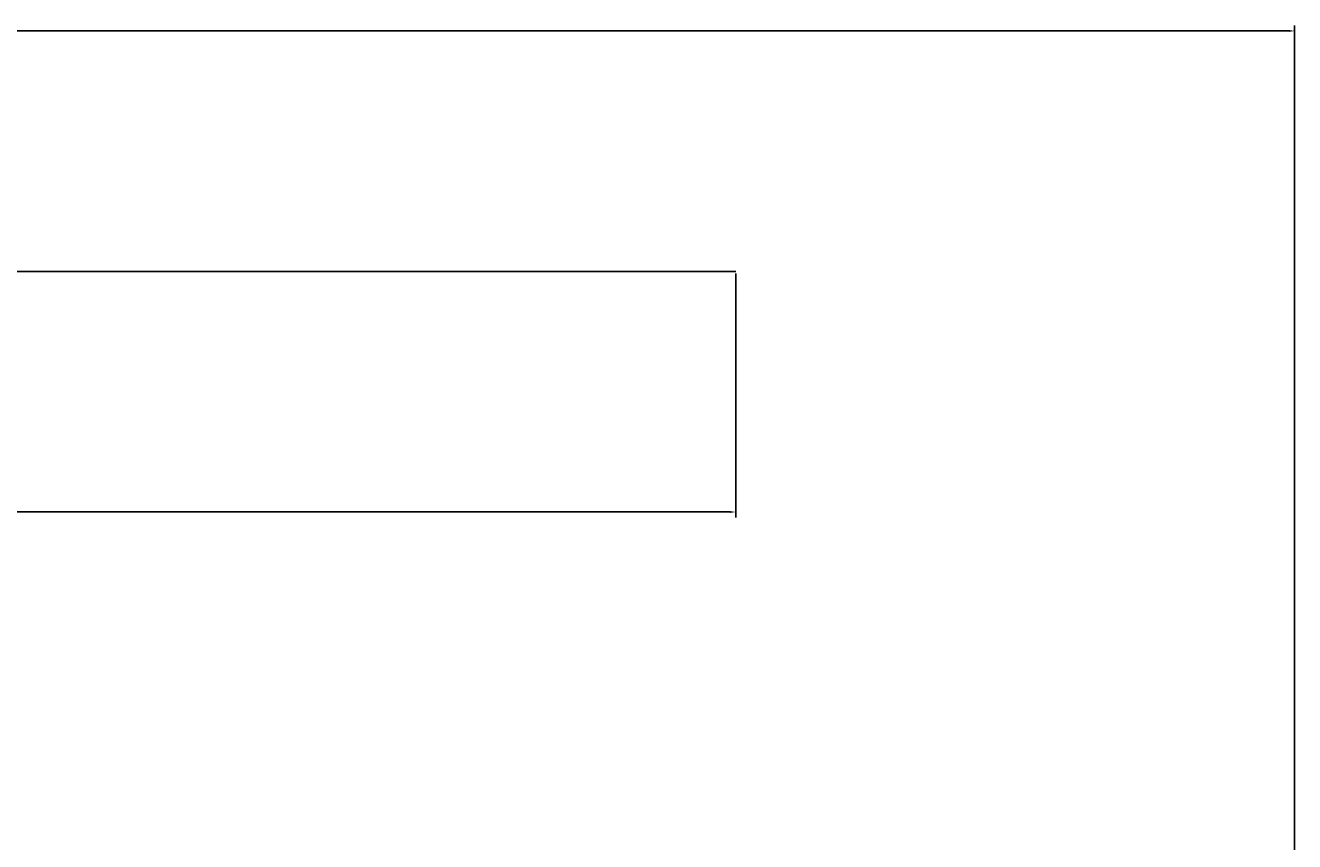
# Model space of a CAD drawing. Units: millimetres. Extents: x 223 to 381, y -8 to 62.
# Tile 5 of 5: x 332 to 373, y 36 to 62. Entities that reach past the tile are written whole.
import ezdxf

# ---------------------------------------------------------------- set-up
doc = ezdxf.new("R2010")
doc.units = ezdxf.units.MM
doc.layers.add('M-CONS', color=8, linetype='Continuous', lineweight=13)
doc.layers.add('M-DIMS', color=2, linetype='Continuous', lineweight=18)
doc.styles.get("Standard").update_dxf_attribs({"font": 'arial.ttf'})
doc.dimstyles.get("Standard").update_dxf_attribs({"dimtxt": 0.18, "dimasz": 0.18, "dimexe": 0.18, "dimexo": 0.0625, "dimgap": 0.09, "dimtad": 0, "dimtih": 1, "dimtoh": 1, "dimdec": 4, "dimzin": 0, "dimdsep": 46, "dimtxsty": 'Standard', "dimcen": 0.09, "dimadec": 0, "dimazin": 0, "dimtfac": 1, "dimtdec": 4, "dimtofl": 0, "dimtmove": 0, "dimatfit": 3, "dimfxl": 1, "dimtolj": 1, "dimtzin": 0, "dimarcsym": 0})

# ---------------------------------------------------------------- blocks, each defined once
blk = doc.blocks.new('*D1')
at = {"layer": 'Defpoints', "color": 0, "transparency": 16777216}
for p in [(372.659, 61.75), (372.659, 27), (230.659, 0)]:
    blk.add_point(p, dxfattribs=at)
at = {"layer": 'M-DIMS', "color": 0, "lineweight": -2, "transparency": 16777216}
for p, q in [((230.659, 0.062), (230.659, 61.93)), ((230.839, 61.75), (301.38, 61.75)), ((372.479, 61.75), (301.939, 61.75)), ((372.659, 27.062), (372.659, 61.93))]:
    blk.add_line(p, q, dxfattribs=at)
at = {"layer": 'M-DIMS', "color": 0, "transparency": 16777216}
for points in [[(230.839, 61.78), (230.839, 61.72), (230.659, 61.75)], [(372.479, 61.78), (372.479, 61.72), (372.659, 61.75)]]:
    blk.add_solid(points, dxfattribs=at)
at = {"layer": 'M-DIMS', "color": 0, "transparency": 16777216, "insert": (301.659, 61.75), "char_height": 0.18, "attachment_point": 5}
blk.add_mtext('\\A1;142', dxfattribs=at)
blk = doc.blocks.new('*D7')
at = {"layer": 'Defpoints', "color": 0, "transparency": 16777216}
for p in [(294.659, 54), (354.659, 54), (294.659, 46.25)]:
    blk.add_point(p, dxfattribs=at)
at = {"layer": 'M-DIMS', "color": 0, "lineweight": -2, "transparency": 16777216}
for p, q in [((294.659, 53.938), (294.659, 46.07)), ((354.659, 53.938), (354.659, 46.07)), ((294.839, 46.25), (324.44, 46.25)), ((354.479, 46.25), (324.878, 46.25))]:
    blk.add_line(p, q, dxfattribs=at)
at = {"layer": 'M-DIMS', "color": 0, "transparency": 16777216}
for points in [[(294.839, 46.28), (294.839, 46.22), (294.659, 46.25)], [(354.479, 46.28), (354.479, 46.22), (354.659, 46.25)]]:
    blk.add_solid(points, dxfattribs=at)
at = {"layer": 'M-DIMS', "color": 0, "transparency": 16777216, "insert": (324.659, 46.25), "char_height": 0.18, "attachment_point": 5}
blk.add_mtext('\\A1;60', dxfattribs=at)

msp = doc.modelspace()

# ---------------------------------------------------------------- linework, layer by layer
at = {"layer": 'M-CONS', "extrusion": (0, -1, 0), "elevation": -54}
msp.add_lwpolyline([(294.6592, 85.6363), (354.6592, 85.6363), (354.6592, 63.6363), (294.6592, 63.6363)], close=True, dxfattribs=at)

# ---------------------------------------------------------------- dimensions: what is measured, and where the dimension line sits
at = {"layer": 'M-DIMS'}
dim = msp.add_linear_dim(base=(372.6592, 61.75), p1=(230.6592, 0), p2=(372.6592, 27), dimstyle='Standard', override={"dimdec": 0, "dimlfac": 1, "dimrnd": 0, "dimzin": 0, "dimdsep": 46, "dimlunit": 2}, dxfattribs=at)
dim.commit()
dim.dimension.update_dxf_attribs({"geometry": '*D1', "text_midpoint": (301.6592, 61.75)})
dim = msp.add_linear_dim(base=(294.6592, 46.25), p1=(354.6592, 54), p2=(294.6592, 54), angle=180, dimstyle='Standard', override={"dimdec": 0, "dimlfac": 1, "dimrnd": 0, "dimzin": 0, "dimdsep": 46, "dimlunit": 2}, dxfattribs=at)
dim.commit()
dim.dimension.update_dxf_attribs({"geometry": '*D7', "text_midpoint": (324.6592, 46.25)})

doc.saveas('drawing.dxf')
